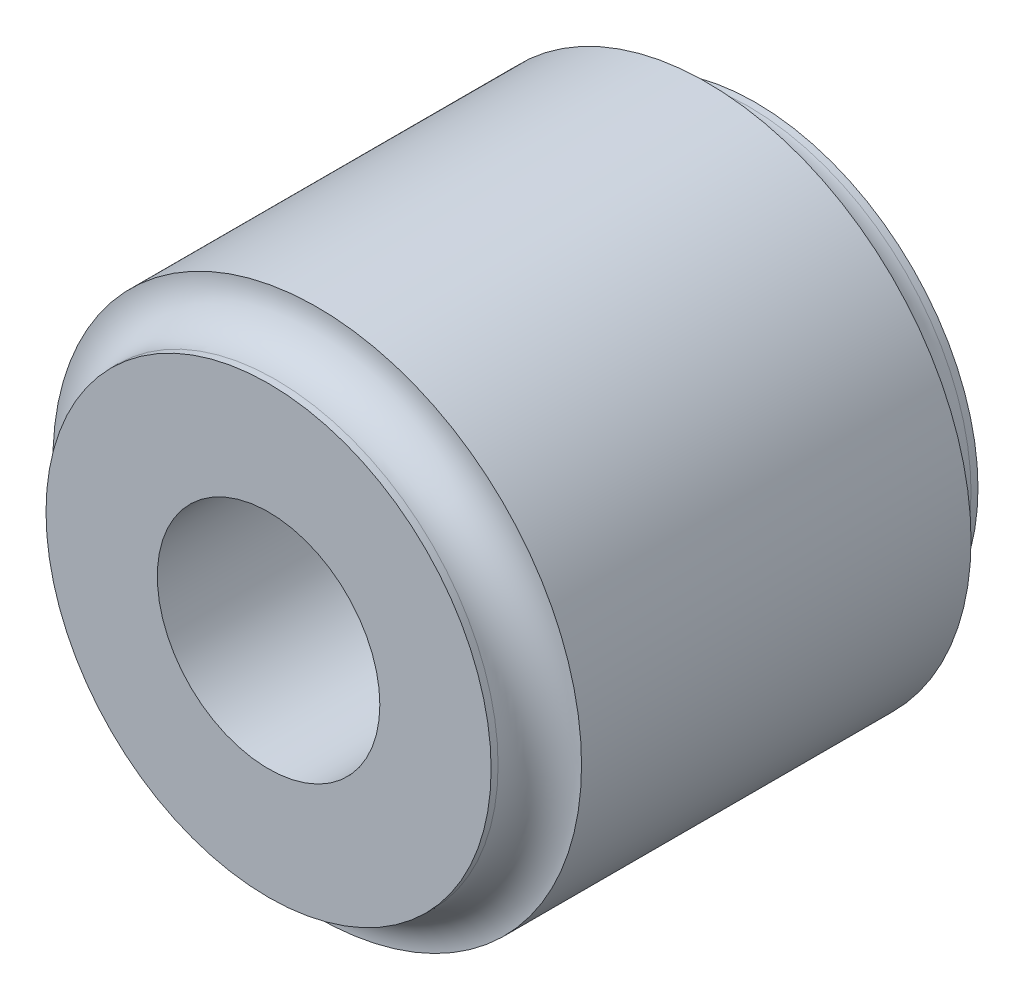
ISO-10303-21;
HEADER;
FILE_DESCRIPTION(('STEP AP214'),'2;1');
FILE_NAME('part.step','',(''),(''),'','','');
FILE_SCHEMA(('AUTOMOTIVE_DESIGN { 1 0 10303 214 1 1 1 1 }'));
ENDSEC;
DATA;
#1=APPLICATION_CONTEXT('core data for automotive mechanical design processes');
#2=APPLICATION_PROTOCOL_DEFINITION('international standard','automotive_design',2000,#1);
#3=PRODUCT_CONTEXT('',#1,'mechanical');
#4=PRODUCT('Part','Part','',(#3));
#5=PRODUCT_RELATED_PRODUCT_CATEGORY('part','',(#4));
#6=PRODUCT_DEFINITION_FORMATION('','',#4);
#7=PRODUCT_DEFINITION_CONTEXT('part definition',#1,'design');
#8=PRODUCT_DEFINITION('design','',#6,#7);
#9=PRODUCT_DEFINITION_SHAPE('','',#8);
#10=(LENGTH_UNIT() NAMED_UNIT(*) SI_UNIT(.MILLI.,.METRE.));
#11=(NAMED_UNIT(*) PLANE_ANGLE_UNIT() SI_UNIT($,.RADIAN.));
#12=(NAMED_UNIT(*) SI_UNIT($,.STERADIAN.) SOLID_ANGLE_UNIT());
#13=UNCERTAINTY_MEASURE_WITH_UNIT(LENGTH_MEASURE(1.E-05),#10,'distance_accuracy_value','');
#14=(GEOMETRIC_REPRESENTATION_CONTEXT(3) GLOBAL_UNCERTAINTY_ASSIGNED_CONTEXT((#13)) GLOBAL_UNIT_ASSIGNED_CONTEXT((#10,
#11,#12)) REPRESENTATION_CONTEXT('',''));
#15=CARTESIAN_POINT('',(0.,0.,0.));
#16=DIRECTION('',(0.,0.,1.));
#17=DIRECTION('',(1.,0.,0.));
#18=AXIS2_PLACEMENT_3D('',#15,#16,#17);
#19=CARTESIAN_POINT('',(0.,0.,14.));
#20=DIRECTION('',(0.,0.,-1.));
#21=DIRECTION('',(-1.,0.,0.));
#22=AXIS2_PLACEMENT_3D('',#19,#20,#21);
#23=CYLINDRICAL_SURFACE('',#22,19.);
#24=CARTESIAN_POINT('',(0.,0.,14.));
#25=DIRECTION('',(0.,0.,1.));
#26=DIRECTION('',(1.,0.,0.));
#27=AXIS2_PLACEMENT_3D('',#24,#25,#26);
#28=CIRCLE('',#27,19.);
#29=CARTESIAN_POINT('',(19.,0.,14.));
#30=VERTEX_POINT('',#29);
#31=EDGE_CURVE('E48',#30,#30,#28,.T.);
#32=ORIENTED_EDGE('',*,*,#31,.F.);
#33=EDGE_LOOP('',(#32));
#34=FACE_BOUND('',#33,.T.);
#35=CARTESIAN_POINT('',(0.,0.,-14.));
#36=DIRECTION('',(0.,0.,1.));
#37=DIRECTION('',(1.,0.,0.));
#38=AXIS2_PLACEMENT_3D('',#35,#36,#37);
#39=CIRCLE('',#38,19.);
#40=CARTESIAN_POINT('',(19.,0.,-14.));
#41=VERTEX_POINT('',#40);
#42=EDGE_CURVE('E55',#41,#41,#39,.T.);
#43=ORIENTED_EDGE('',*,*,#42,.T.);
#44=EDGE_LOOP('',(#43));
#45=FACE_BOUND('',#44,.T.);
#46=ADVANCED_FACE('F40',(#34,#45),#23,.T.);
#47=CARTESIAN_POINT('',(0.,0.,-17.5));
#48=DIRECTION('',(0.,0.,1.));
#49=DIRECTION('',(1.,0.,0.));
#50=AXIS2_PLACEMENT_3D('',#47,#48,#49);
#51=PLANE('',#50);
#52=CARTESIAN_POINT('',(0.,0.,-17.5));
#53=DIRECTION('',(0.,0.,1.));
#54=DIRECTION('',(1.,0.,0.));
#55=AXIS2_PLACEMENT_3D('',#52,#53,#54);
#56=CIRCLE('',#55,8.);
#57=CARTESIAN_POINT('',(8.,0.,-17.5));
#58=VERTEX_POINT('',#57);
#59=EDGE_CURVE('E61',#58,#58,#56,.T.);
#60=ORIENTED_EDGE('',*,*,#59,.T.);
#61=EDGE_LOOP('',(#60));
#62=FACE_BOUND('',#61,.T.);
#63=CARTESIAN_POINT('',(0.,0.,-17.5));
#64=DIRECTION('',(0.,0.,1.));
#65=DIRECTION('',(1.,0.,0.));
#66=AXIS2_PLACEMENT_3D('',#63,#64,#65);
#67=CIRCLE('',#66,16.);
#68=CARTESIAN_POINT('',(16.,0.,-17.5));
#69=VERTEX_POINT('',#68);
#70=EDGE_CURVE('E59',#69,#69,#67,.T.);
#71=ORIENTED_EDGE('',*,*,#70,.F.);
#72=EDGE_LOOP('',(#71));
#73=FACE_BOUND('',#72,.T.);
#74=ADVANCED_FACE('F66',(#62,#73),#51,.F.);
#75=CARTESIAN_POINT('',(0.,0.,17.5));
#76=DIRECTION('',(0.,0.,-1.));
#77=DIRECTION('',(-1.,0.,0.));
#78=AXIS2_PLACEMENT_3D('',#75,#76,#77);
#79=CYLINDRICAL_SURFACE('',#78,16.);
#80=CARTESIAN_POINT('',(0.,0.,-17.));
#81=DIRECTION('',(0.,0.,1.));
#82=DIRECTION('',(1.,0.,0.));
#83=AXIS2_PLACEMENT_3D('',#80,#81,#82);
#84=CIRCLE('',#83,16.);
#85=CARTESIAN_POINT('',(16.,0.,-17.));
#86=VERTEX_POINT('',#85);
#87=EDGE_CURVE('E42',#86,#86,#84,.F.);
#88=ORIENTED_EDGE('',*,*,#87,.T.);
#89=EDGE_LOOP('',(#88));
#90=FACE_BOUND('',#89,.T.);
#91=ORIENTED_EDGE('',*,*,#70,.T.);
#92=EDGE_LOOP('',(#91));
#93=FACE_BOUND('',#92,.T.);
#94=ADVANCED_FACE('F86',(#90,#93),#79,.T.);
#95=CARTESIAN_POINT('',(0.,0.,17.));
#96=DIRECTION('',(0.,0.,1.));
#97=DIRECTION('',(1.,0.,0.));
#98=AXIS2_PLACEMENT_3D('',#95,#96,#97);
#99=CIRCLE('',#98,16.);
#100=CARTESIAN_POINT('',(16.,0.,17.));
#101=VERTEX_POINT('',#100);
#102=EDGE_CURVE('E10',#101,#101,#99,.T.);
#103=ORIENTED_EDGE('',*,*,#102,.T.);
#104=EDGE_LOOP('',(#103));
#105=FACE_BOUND('',#104,.T.);
#106=CARTESIAN_POINT('',(0.,0.,17.5));
#107=DIRECTION('',(0.,0.,1.));
#108=DIRECTION('',(1.,0.,0.));
#109=AXIS2_PLACEMENT_3D('',#106,#107,#108);
#110=CIRCLE('',#109,16.);
#111=CARTESIAN_POINT('',(16.,0.,17.5));
#112=VERTEX_POINT('',#111);
#113=EDGE_CURVE('E57',#112,#112,#110,.T.);
#114=ORIENTED_EDGE('',*,*,#113,.F.);
#115=EDGE_LOOP('',(#114));
#116=FACE_BOUND('',#115,.T.);
#117=ADVANCED_FACE('F83',(#105,#116),#79,.T.);
#118=CARTESIAN_POINT('',(0.,0.,17.5));
#119=DIRECTION('',(0.,0.,1.));
#120=DIRECTION('',(1.,0.,0.));
#121=AXIS2_PLACEMENT_3D('',#118,#119,#120);
#122=PLANE('',#121);
#123=CARTESIAN_POINT('',(0.,0.,17.5));
#124=DIRECTION('',(0.,0.,1.));
#125=DIRECTION('',(1.,0.,0.));
#126=AXIS2_PLACEMENT_3D('',#123,#124,#125);
#127=CIRCLE('',#126,8.);
#128=CARTESIAN_POINT('',(8.,0.,17.5));
#129=VERTEX_POINT('',#128);
#130=EDGE_CURVE('E63',#129,#129,#127,.T.);
#131=ORIENTED_EDGE('',*,*,#130,.F.);
#132=EDGE_LOOP('',(#131));
#133=FACE_BOUND('',#132,.T.);
#134=ORIENTED_EDGE('',*,*,#113,.T.);
#135=EDGE_LOOP('',(#134));
#136=FACE_BOUND('',#135,.T.);
#137=ADVANCED_FACE('F78',(#133,#136),#122,.T.);
#138=CARTESIAN_POINT('',(0.,0.,-17.));
#139=DIRECTION('',(0.,0.,1.));
#140=DIRECTION('',(1.,0.,0.));
#141=AXIS2_PLACEMENT_3D('',#138,#139,#140);
#142=TOROIDAL_SURFACE('',#141,19.,3.);
#143=ORIENTED_EDGE('',*,*,#42,.F.);
#144=EDGE_LOOP('',(#143));
#145=FACE_BOUND('',#144,.T.);
#146=ORIENTED_EDGE('',*,*,#87,.F.);
#147=EDGE_LOOP('',(#146));
#148=FACE_BOUND('',#147,.T.);
#149=ADVANCED_FACE('F85',(#145,#148),#142,.F.);
#150=CARTESIAN_POINT('',(0.,0.,17.));
#151=DIRECTION('',(0.,0.,1.));
#152=DIRECTION('',(1.,0.,0.));
#153=AXIS2_PLACEMENT_3D('',#150,#151,#152);
#154=TOROIDAL_SURFACE('',#153,19.,3.);
#155=ORIENTED_EDGE('',*,*,#102,.F.);
#156=EDGE_LOOP('',(#155));
#157=FACE_BOUND('',#156,.T.);
#158=ORIENTED_EDGE('',*,*,#31,.T.);
#159=EDGE_LOOP('',(#158));
#160=FACE_BOUND('',#159,.T.);
#161=ADVANCED_FACE('F39',(#157,#160),#154,.F.);
#162=CARTESIAN_POINT('',(0.,0.,-17.5));
#163=DIRECTION('',(0.,0.,1.));
#164=DIRECTION('',(1.,0.,0.));
#165=AXIS2_PLACEMENT_3D('',#162,#163,#164);
#166=CYLINDRICAL_SURFACE('',#165,8.);
#167=ORIENTED_EDGE('',*,*,#59,.F.);
#168=EDGE_LOOP('',(#167));
#169=FACE_BOUND('',#168,.T.);
#170=ORIENTED_EDGE('',*,*,#130,.T.);
#171=EDGE_LOOP('',(#170));
#172=FACE_BOUND('',#171,.T.);
#173=ADVANCED_FACE('F71',(#169,#172),#166,.F.);
#174=CLOSED_SHELL('',(#46,#74,#94,#117,#137,#149,#161,#173));
#175=MANIFOLD_SOLID_BREP('B2',#174);
#176=ADVANCED_BREP_SHAPE_REPRESENTATION('',(#18,#175),#14);
#177=SHAPE_DEFINITION_REPRESENTATION(#9,#176);
ENDSEC;
END-ISO-10303-21;
